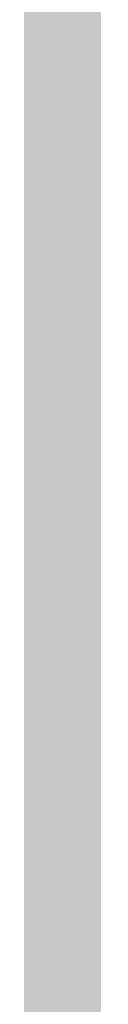
# Model space of a CAD drawing. Units: inches. Extents: x 2083 to 3317, y 1141 to 2115.
# Tile 228 of 256: x 3126.67 to 3126.939, y 1267.234 to 1271.372. Entities that reach past the tile are written whole.
import ezdxf

# ---------------------------------------------------------------- set-up
doc = ezdxf.new("R2010")
doc.units = ezdxf.units.IN
doc.layers.add('A-ANNO-DIMS', color=2, linetype='Continuous', lineweight=18)
doc.layers.add('A-WALL-PATT', color=251, linetype='Continuous', lineweight=13, true_color=0x636466)
doc.styles.get("Standard").update_dxf_attribs({"font": 'arial.ttf'})
doc.dimstyles.new('ISO-25', dxfattribs={"dimtxt": 12, "dimasz": 12, "dimexe": 1.25, "dimexo": 0.625, "dimtad": 1, "dimlunit": 3, "dimtxsty": 'Standard', "dimcen": 2.5, "dimadec": 0, "dimazin": 0, "dimtfac": 1, "dimtmove": 0, "dimatfit": 3, "dimfxl": 1, "dimarcsym": 0})

# ---------------------------------------------------------------- blocks, each defined once
blk = doc.blocks.new('*D26')
at = {"layer": 'A-ANNO-DIMS', "color": 0, "lineweight": -2, "transparency": 16777216}
for p, q in [((3088.9858, 1274.9151), (3088.9858, 1270.952)), ((3111.24, 1274.9151), (3111.24, 1270.952)), ((3076.9858, 1272.202), (2840.2624, 1272.202)), ((3111.24, 1272.202), (3088.9858, 1272.202)), ((3123.24, 1272.202), (3135.24, 1272.202))]:
    blk.add_line(p, q, dxfattribs=at)
at = {"layer": 'A-ANNO-DIMS', "color": 0, "transparency": 16777216}
for points in [[(3076.9858, 1274.202), (3076.9858, 1270.202), (3088.9858, 1272.202)], [(3123.24, 1274.202), (3123.24, 1270.202), (3111.24, 1272.202)]]:
    blk.add_solid(points, dxfattribs=at)
at = {"layer": 'Defpoints', "color": 0, "transparency": 16777216}
for p in [(3088.9858, 1275.5401), (3111.24, 1275.5401), (3088.9858, 1272.202)]:
    blk.add_point(p, dxfattribs=at)
at = {"layer": 'A-ANNO-DIMS', "color": 0, "transparency": 16777216, "insert": (2952.6241, 1279.0316), "char_height": 12, "attachment_point": 5}
blk.add_mtext('NIGHTSTAND 1\'-10 1/2" TYP.', dxfattribs=at)
blk = doc.blocks.new('*D27')
at = {"layer": 'A-ANNO-DIMS', "color": 0, "lineweight": -2, "transparency": 16777216}
for p, q in [((3114.5782, 1309.7943), (3114.5782, 1321.7943)), ((3111.865, 1297.7943), (3115.8282, 1297.7943)), ((3114.5782, 1297.7943), (3114.5782, 1275.5401)), ((3111.865, 1275.5401), (3115.8282, 1275.5401)), ((3114.5782, 1263.5401), (3114.5782, 1140.9886))]:
    blk.add_line(p, q, dxfattribs=at)
at = {"layer": 'A-ANNO-DIMS', "color": 0, "transparency": 16777216}
for points in [[(3112.5782, 1309.7943), (3116.5782, 1309.7943), (3114.5782, 1297.7943)], [(3112.5782, 1263.5401), (3116.5782, 1263.5401), (3114.5782, 1275.5401)]]:
    blk.add_solid(points, dxfattribs=at)
at = {"layer": 'Defpoints', "color": 0, "transparency": 16777216}
for p in [(3111.24, 1297.7943), (3111.24, 1275.5401), (3114.5782, 1275.5401)]:
    blk.add_point(p, dxfattribs=at)
at = {"layer": 'A-ANNO-DIMS', "color": 0, "transparency": 16777216, "insert": (3107.7485, 1196.2643), "char_height": 12, "attachment_point": 5, "rotation": 90}
blk.add_mtext('1\'-10 1/2" TYP.', dxfattribs=at)

msp = doc.modelspace()

# ---------------------------------------------------------------- hatches: boundary and pattern name
at = {"layer": 'A-WALL-PATT'}
h = msp.add_hatch(color=256, dxfattribs=at)
h.dxf.hatch_style = 1
h.paths.add_polyline_path([(3126.9598, 2020.7614), (2748.9598, 2020.7614), (2604.9598, 2020.7614), (2226.9598, 2020.7614), (2226.9598, 1702.7614), (2466.9598, 1702.7614), (2466.9598, 1582.7614), (2418.9598, 1582.7614), (2418.9598, 1477.7614), (2226.9598, 1477.7614), (2226.9598, 1263.2614), (2544.9598, 1263.2614), (2544.9598, 1411.7614), (2604.9598, 1411.7614), (2685.9598, 1411.7614), (2685.9598, 1420.7614), (2604.9598, 1420.7614), (2604.9598, 1573.7614), (2604.9598, 1702.7614), (2604.9598, 2011.7614), (2748.9598, 2011.7614), (2748.9598, 1702.7614), (2862.9598, 1702.7614), (2862.9598, 1621.7614), (2871.9598, 1621.7614), (2871.9598, 1702.7614), (2883.9598, 1702.7614), (2883.9598, 1706.9395, -0.026459), (2883.9598, 1711.7614), (2757.9598, 1711.7614), (2757.9598, 1807.7614), (2787.9598, 1807.7614), (2787.9598, 1812.2614), (2757.9598, 1812.2614), (2757.9598, 2011.7614), (2877.9598, 2011.7614), (2877.9598, 1812.2614), (2847.9598, 1812.2614), (2847.9598, 1807.7614), (2889.8357, 1807.7614), (2889.8357, 1812.2614), (2882.4598, 1812.2614), (2882.4598, 2011.7614), (3117.9598, 2011.7614), (3117.9598, 1812.2614), (2937.8357, 1812.2614), (2937.8357, 1807.7614), (2995.7098, 1807.7614), (2995.7098, 1796.1177), (3000.2098, 1796.1177), (3000.2098, 1807.7614), (3117.9598, 1807.7614), (3117.9598, 1711.7614), (3000.2098, 1711.7614), (3000.2098, 1760.1177), (2998.5727, 1760.1177, -0.020711), (2995.7098, 1760.1177), (2995.7098, 1711.7614), (2931.9598, 1711.7614), (2931.9598, 1702.7614), (3126.9598, 1702.7614)])
h.paths.add_polyline_path([(2471.4598, 2011.7614), (2471.4598, 1810.0114), (2462.7169, 1810.0114), (2462.7169, 1805.5114), (2505.9598, 1805.5114), (2505.9598, 1810.0114), (2475.9598, 1810.0114), (2475.9598, 2011.7614), (2595.9598, 2011.7614), (2595.9598, 1810.0114), (2565.9598, 1810.0114), (2565.9598, 1805.5114), (2595.9598, 1805.5114), (2595.9598, 1711.7614), (2235.9598, 1711.7614), (2235.9598, 1805.5114), (2353.7098, 1805.5114), (2353.7098, 1796.0542), (2358.2098, 1796.0542), (2358.2098, 1805.5114), (2414.7169, 1805.5114), (2414.7169, 1810.0114), (2235.9598, 1810.0114), (2235.9598, 2011.7614)], flags=16)
h.paths.add_polyline_path([(2270.2047, 1994.61), (2270.2047, 1970.61), (2246.2047, 1970.61), (2246.2047, 1994.61)], flags=0)
edge = h.paths.add_edge_path(flags=0)
edge.add_ellipse((2332.0274, 1899.7982), major_axis=(-3.043, 3.043), ratio=0.168252, start_angle=-161.3322, end_angle=-156.3071, ccw=False)
edge.add_ellipse((2333.082, 1898.7435), major_axis=(-1.0546, 1.0546), ratio=0.453532, start_angle=-123.371, end_angle=-94.1591)
edge = h.paths.add_edge_path(flags=0)
edge.add_ellipse((2332.0274, 1968.8763), major_axis=(3.043, 3.043), ratio=0.168252, start_angle=18.6678, end_angle=23.6929)
edge.add_spline(control_points=[(2332.9256, 1970.6911), (2332.2268, 1970.3361), (2330.8937, 1969.6589), (2328.4131, 1970.9321), (2327.2039, 1967.7487), (2324.7096, 1969.9556), (2322.5328, 1967.0124), (2320.0128, 1971.2958), (2317.6803, 1968.1578), (2316.0405, 1967.102), (2315.4269, 1966.8096)], knot_values=[0, 0, 0, 0, 2.267059, 4.324559, 6.685584, 8.878641, 11.121502, 14.300359, 17.755284, 19.732645, 19.732645, 19.732645, 19.732645], degree=3, periodic=0)
edge.add_ellipse((2332.0274, 1968.8763), major_axis=(3.043, 3.043), ratio=0.168252, start_angle=18.6678, end_angle=23.6929, ccw=False)
edge.add_ellipse((2333.082, 1969.9309), major_axis=(1.0546, 1.0546), ratio=0.453532, start_angle=56.629, end_angle=85.8409, ccw=False)
edge = h.paths.add_edge_path(flags=0)
edge.add_spline(control_points=[(2296.4283, 1967.9879), (2293.6278, 1965.3363), (2287.7036, 1959.7271), (2299.7439, 1949.9957), (2294.5326, 1935.6685), (2290.5732, 1920.6035), (2293.3941, 1909.9737), (2296.1854, 1904.9665)], knot_values=[0.099185, 0.099185, 0.099185, 0.099185, 0.345301, 0.619822, 0.982653, 1.386093, 1.810555, 1.810555, 1.810555, 1.810555], degree=3, periodic=0)
edge.add_spline(control_points=[(2296.1854, 1904.9665), (2297.3836, 1902.6193), (2298.001, 1901.9493), (2298.553, 1901.4682)], knot_values=[0.006246, 0.006246, 0.006246, 0.006246, 0.055476, 0.055476, 0.055476, 0.055476], degree=3, periodic=0)
edge.add_spline(control_points=[(2298.553, 1901.4682), (2297.2586, 1900.9232), (2295.2253, 1900.2321), (2293.0602, 1900.6142), (2292.1014, 1900.7884), (2292.0896, 1900.7906)], knot_values=[0.312835, 0.312835, 0.312835, 0.312835, 0.40178, 0.474987, 0.475903, 0.475903, 0.475903, 0.475903], degree=3, periodic=0)
edge.add_arc((2292.7936, 1904.6641), 3.937, 215.4209, 259.6982, ccw=False)
edge.add_spline(control_points=[(2289.5853, 1902.3823), (2289.4767, 1902.5351), (2289.3685, 1902.688), (2289.2609, 1902.8412)], knot_values=[0.102872, 0.102872, 0.102872, 0.102872, 0.116896, 0.116896, 0.116896, 0.116896], degree=3, periodic=0)
edge.add_spline(control_points=[(2289.2609, 1902.8412), (2288.6866, 1902.5502), (2287.64, 1902.0199), (2285.8813, 1901.874), (2283.853, 1901.5044), (2281.72, 1899.7105), (2278.467, 1899.4929), (2276.1571, 1901.8832), (2272.259, 1899.8041), (2267.7776, 1901.8432), (2262.2439, 1900.184), (2257.4149, 1901.7821), (2254.3184, 1900.7261), (2253.1783, 1900.3373)], knot_values=[0, 0, 0, 0, 1.907977, 3.477176, 5.261074, 7.972851, 11.680248, 13.717921, 16.939592, 22.789562, 27.502503, 33.595215, 37.145618, 37.145618, 37.145618, 37.145618], degree=3, periodic=0)
edge.add_line((2253.1783, 1900.3373), (2250.2442, 1902.8412))
edge.add_line((2250.2442, 1902.8412), (2250.2442, 1965.8333))
edge.add_line((2250.2442, 1965.8333), (2253.1783, 1968.3371))
edge.add_spline(control_points=[(2253.1783, 1968.3371), (2254.3184, 1967.9483), (2257.4149, 1966.8924), (2262.2439, 1968.4904), (2267.7776, 1966.8313), (2271.5267, 1968.5372), (2273.8759, 1967.8283), (2274.2067, 1967.7276)], knot_values=[0, 0, 0, 0, 0.09018, 0.244935, 0.364644, 0.513233, 0.537855, 0.537855, 0.537855, 0.537855], degree=3, periodic=0)
edge.add_arc((2274.3529, 1963.7933), 3.937, 72.0511, 92.1279, ccw=False)
edge.add_arc((2281.2969, 1985.23), 18.5963, 252.05113, 288.56572)
edge.add_arc((2292.3167, 1956.0289), 12.6461, 71.02679, 113.77822, ccw=False)
edge = h.paths.add_edge_path(flags=0)
edge.add_spline(control_points=[(2274.8994, 1951.8562), (2275.0662, 1951.6166), (2275.2327, 1951.3766), (2275.398, 1951.1359)], knot_values=[1.409916, 1.409916, 1.409916, 1.409916, 1.43159, 1.43159, 1.43159, 1.43159], degree=3, periodic=0)
edge.add_spline(control_points=[(2275.398, 1951.1359), (2275.7921, 1950.5619), (2276.1792, 1949.9838), (2276.5455, 1949.3971)], knot_values=[1.358238, 1.358238, 1.358238, 1.358238, 1.409916, 1.409916, 1.409916, 1.409916], degree=3, periodic=0)
edge.add_line((2276.5455, 1949.3971), (2277.4373, 1947.8622))
edge.add_spline(control_points=[(2277.4373, 1947.8622), (2276.3038, 1945.6731), (2274.6397, 1942.4269), (2274.6316, 1938.0939), (2272.7991, 1930.8515), (2274.3564, 1943.897), (2275.9477, 1947.9234), (2276.5455, 1949.3971)], knot_values=[0.005632, 0.005632, 0.005632, 0.005632, 0.186014, 0.266002, 0.357087, 0.59639, 0.739732, 0.739732, 0.739732, 0.739732], degree=3, periodic=0)
edge.add_spline(control_points=[(2276.5455, 1949.3971), (2276.1792, 1949.9838), (2275.7921, 1950.5619), (2275.398, 1951.1359)], knot_values=[1.358238, 1.358238, 1.358238, 1.358238, 1.409916, 1.409916, 1.409916, 1.409916], degree=3, periodic=0)
edge.add_spline(control_points=[(2275.398, 1951.1359), (2274.9425, 1950.0805), (2274.2078, 1948.0253), (2273.9346, 1944.8515), (2272.4685, 1937.6275), (2273.4662, 1945.6965), (2274.7006, 1951.0595), (2274.8994, 1951.8562)], knot_values=[0.104364, 0.104364, 0.104364, 0.104364, 0.189636, 0.269624, 0.36071, 0.600013, 0.644622, 0.644622, 0.644622, 0.644622], degree=3, periodic=0)
h.paths.add_polyline_path([(2269.1675, 1963.1276, -0.357527), (2268.1706, 1960.9764, -0.092561), (2268.1706, 1939.4363, -0.357527), (2269.1675, 1937.2851, -0.357527), (2267.0163, 1938.282, -0.164785), (2254.6856, 1938.282, -0.357527), (2252.5344, 1937.2851, -0.357527), (2253.5313, 1939.4363, -0.092561), (2253.5313, 1960.9764, -0.357527), (2252.5344, 1963.1276, -0.357527), (2254.6856, 1962.1307, -0.164785), (2267.0163, 1962.1307, -0.357527)], flags=0)
h.paths.add_polyline_path([(2248.8741, 1967.8018), (2248.8741, 1957.0277), (2249.4578, 1957.0277), (2249.4578, 1911.6468), (2248.8741, 1911.6468), (2248.8741, 1900.8727), (2246.5119, 1900.8727, 0.197327), (2244.1497, 1902.4569), (2244.1497, 1966.2176, 0.197327), (2246.5119, 1967.8018)], flags=0)
h.paths.add_polyline_path([(2269.1675, 1931.3893, -0.357527), (2268.1706, 1929.2381, -0.092561), (2268.1706, 1907.6981, -0.357527), (2269.1675, 1905.5469, -0.357527), (2267.0163, 1906.5438, -0.164785), (2254.6856, 1906.5438, -0.357527), (2252.5344, 1905.5469, -0.357527), (2253.5313, 1907.6981, -0.092561), (2253.5313, 1929.2381, -0.357527), (2252.5344, 1931.3893, -0.357527), (2254.6856, 1930.3925, -0.164785), (2267.0163, 1930.3925, -0.357527)], flags=0)
edge = h.paths.add_edge_path(flags=0)
edge.add_spline(control_points=[(2276.1969, 1906.7237), (2276.1681, 1909.0289), (2276.114, 1913.3719), (2270.5984, 1924.925), (2273.9052, 1919.0128), (2275.9217, 1916.2621), (2275.4746, 1912.4021), (2277.2579, 1910.3806), (2276.696, 1908.225), (2276.6462, 1906.813), (2276.6178, 1906.0084)], knot_values=[0, 0, 0, 0, 8.61026, 16.221274, 18.843057, 23.804898, 27.440828, 29.356102, 31.203478, 33.650687, 33.650687, 33.650687, 33.650687], degree=3, periodic=0)
edge.add_spline(control_points=[(2276.6178, 1906.0084), (2276.6233, 1905.6241), (2276.4977, 1904.6287), (2275.4418, 1903.8547), (2274.9373, 1903.0804), (2274.8591, 1902.8412)], knot_values=[0.156488, 0.156488, 0.156488, 0.156488, 0.184398, 0.231376, 0.250598, 0.250598, 0.250598, 0.250598], degree=3, periodic=0)
edge.add_line((2274.8591, 1902.8412), (2276.506, 1902.8412))
edge.add_spline(control_points=[(2276.506, 1902.8412), (2276.7883, 1903.0849), (2277.6651, 1904.1252), (2278.2495, 1904.3407), (2277.6539, 1908.5274), (2278.1557, 1906.2278), (2278.1005, 1905.2859), (2278.8467, 1904.069), (2277.8568, 1903.4149), (2277.8742, 1902.991), (2277.9036, 1902.8412)], knot_values=[0.059574, 0.059574, 0.059574, 0.059574, 0.080753, 0.103741, 0.16972, 0.176036, 0.207137, 0.240474, 0.262341, 0.27366, 0.27366, 0.27366, 0.27366], degree=3, periodic=0)
edge.add_line((2277.9036, 1902.8412), (2280.0298, 1902.8412))
edge.add_spline(control_points=[(2280.0298, 1902.8412), (2279.8882, 1903.0884), (2279.4993, 1903.9816), (2280.1523, 1905.9393), (2278.1036, 1909.6578), (2279.7624, 1907.1853), (2280.3279, 1904.8749), (2280.4851, 1903.4896), (2281.4633, 1903.2494), (2281.7583, 1902.9365), (2281.834, 1902.8412)], knot_values=[0.013856, 0.013856, 0.013856, 0.013856, 0.034874, 0.088867, 0.107879, 0.126738, 0.158714, 0.193757, 0.217487, 0.226722, 0.226722, 0.226722, 0.226722], degree=3, periodic=0)
edge.add_spline(control_points=[(2281.834, 1902.8412), (2281.7875, 1902.8267), (2281.647, 1902.783), (2281.3955, 1902.8595), (2281.0881, 1902.9852), (2280.7207, 1903.0609), (2280.3335, 1903.0257), (2280.1248, 1902.8989), (2280.0298, 1902.8412)], knot_values=[0, 0, 0, 0, 0.14413, 0.435517, 0.749276, 1.153046, 1.548371, 1.878348, 1.878348, 1.878348, 1.878348], degree=3, periodic=0)
edge.add_line((2280.0298, 1902.8412), (2277.9036, 1902.8412))
edge.add_spline(control_points=[(2277.9036, 1902.8412), (2277.8929, 1902.7959), (2277.8654, 1902.6796), (2277.6075, 1902.6875), (2277.2741, 1902.8007), (2276.8379, 1902.6198), (2276.5838, 1902.7893), (2276.506, 1902.8412)], knot_values=[0, 0, 0, 0, 0.127189, 0.326199, 0.628009, 1.24357, 1.515331, 1.515331, 1.515331, 1.515331], degree=3, periodic=0)
edge.add_line((2276.506, 1902.8412), (2274.8591, 1902.8412))
edge.add_spline(control_points=[(2274.8591, 1902.8412), (2274.8144, 1902.8986), (2274.7251, 1903.0134), (2274.4935, 1903.119), (2274.2443, 1902.9605), (2273.9371, 1903.1849), (2273.614, 1902.9831), (2273.4083, 1902.883), (2273.3223, 1902.8412)], knot_values=[0, 0, 0, 0, 0.21843, 0.436957, 0.687977, 0.990379, 1.398396, 1.69185, 1.69185, 1.69185, 1.69185], degree=3, periodic=0)
edge.add_spline(control_points=[(2273.3223, 1902.8412), (2273.6167, 1903.4457), (2274.274, 1904.5383), (2276.0272, 1904.5737), (2276.207, 1906.5836), (2276.1969, 1906.7237)], knot_values=[0.012227, 0.012227, 0.012227, 0.012227, 0.059472, 0.106218, 0.134458, 0.134458, 0.134458, 0.134458], degree=3, periodic=0)
h.paths.add_polyline_path([(2270.7761, 1897.7898), (2270.7761, 1873.7898), (2246.7761, 1873.7898), (2246.7761, 1897.7898)], flags=0)
h.paths.add_polyline_path([(2353.7098, 1760.0051), (2353.7098, 1760.0542), (2358.2098, 1760.0542, -0.033729)], flags=0)
h.paths.add_polyline_path([(2321.8191, 1737.5292), (2341.9953, 1737.5292, -0.414214), (2343.2033, 1736.3212), (2343.2033, 1721.0206, -0.414214), (2341.9953, 1719.8127), (2321.8191, 1719.8127, -0.414214), (2320.6112, 1721.0206), (2320.6112, 1736.3212, -0.414214)], flags=0)
h.paths.add_polyline_path([(2324.235, 1736.3212), (2339.5794, 1736.3212, -0.414214), (2341.9953, 1733.9053), (2341.9953, 1725.4497, -0.414214), (2339.5794, 1723.0338), (2333.6806, 1723.0338), (2333.8453, 1722.0455, -0.870646), (2335.4254, 1721.8259, -0.767327), (2333.9227, 1721.4232), (2331.291, 1721.4232, -0.767327), (2329.7883, 1721.8259, -0.870646), (2331.3684, 1722.0455), (2331.5331, 1723.0338), (2324.235, 1723.0338, -0.414214), (2321.8191, 1725.4497), (2321.8191, 1733.9053, -0.414214)], flags=0)
h.paths.add_polyline_path([(2570.4838, 1928.6154), (2589.6838, 1928.6154), (2590.1688, 1928.6154), (2590.1688, 1904.9934), (2570.4838, 1904.9934)], flags=0)
h.paths.add_polyline_path([(2574.4473, 1927.2638, -1), (2572.8288, 1927.2638, -1)], flags=0)
h.paths.add_polyline_path([(2573.0899, 1926.9409), (2573.925, 1927.776), (2574.1477, 1927.5533), (2573.3126, 1926.7182)], flags=0)
h.paths.add_polyline_path([(2578.7791, 1919.7296, -1), (2571.5917, 1919.7296, -1)], flags=0)
h.paths.add_polyline_path([(2578.3854, 1919.7296, -1), (2571.9854, 1919.7296, -1)], flags=0)
h.paths.add_polyline_path([(2331.5958, 1729.4762, -1), (2333.618, 1729.4762, -1)], flags=0)
h.paths.add_polyline_path([(2578.0342, 1927.2638, -1), (2576.4157, 1927.2638, -1)], flags=0)
h.paths.add_polyline_path([(2576.6889, 1927.5311), (2576.9116, 1927.7538), (2577.7467, 1926.9186), (2577.524, 1926.6959)], flags=0)
h.paths.add_polyline_path([(2578.1391, 1909.8595, -1), (2572.2317, 1909.8595, -1)], flags=0)
h.paths.add_polyline_path([(2577.7454, 1909.8595, -1), (2572.6254, 1909.8595, -1)], flags=0)
h.paths.add_polyline_path([(2583.7977, 1927.2638, -1), (2582.1792, 1927.2638, -1)], flags=0)
h.paths.add_polyline_path([(2582.7186, 1927.7538), (2583.5538, 1926.9186), (2583.3311, 1926.6959), (2582.4959, 1927.5311)], flags=0)
h.paths.add_polyline_path([(2582.4959, 1927.5311), (2582.7186, 1927.7538), (2583.5538, 1926.9186), (2583.3311, 1926.6959)], flags=0)
h.paths.add_polyline_path([(2587.7391, 1920.5296, -1), (2581.8317, 1920.5296, -1)], flags=0)
h.paths.add_polyline_path([(2587.3454, 1920.5296, -1), (2582.2254, 1920.5296, -1)], flags=0)
h.paths.add_polyline_path([(2587.3846, 1927.2638, -1), (2585.7661, 1927.2638, -1)], flags=0)
h.paths.add_polyline_path([(2586.082, 1926.9802), (2586.9172, 1927.8154), (2587.1399, 1927.5927), (2586.3047, 1926.7575)], flags=0)
h.paths.add_polyline_path([(2588.3791, 1910.6595, -1), (2581.1917, 1910.6595, -1)], flags=0)
h.paths.add_polyline_path([(2587.9854, 1910.6595, -1), (2581.5854, 1910.6595, -1)], flags=0)
h.paths.add_polyline_path([(2417.1677, 1729.4779), (2437.3439, 1729.4779, -0.414214), (2438.5519, 1728.2699), (2438.5519, 1712.9693, -0.414214), (2437.3439, 1711.7614), (2417.1677, 1711.7614, -0.414214), (2415.9598, 1712.9693), (2415.9598, 1728.2699, -0.414214)], flags=0)
h.paths.add_polyline_path([(2419.5836, 1728.2699), (2434.928, 1728.2699, -0.414214), (2437.3439, 1725.8541), (2437.3439, 1717.3984, -0.414214), (2434.928, 1714.9825), (2429.0292, 1714.9825), (2429.1939, 1713.9942, -0.870646), (2430.774, 1713.7746, -0.767327), (2429.2713, 1713.372), (2426.6396, 1713.372, -0.767327), (2425.1369, 1713.7746, -0.870646), (2426.717, 1713.9942), (2426.8817, 1714.9825), (2419.5836, 1714.9825, -0.414214), (2417.1677, 1717.3984), (2417.1677, 1725.8541, -0.414214)], flags=0)
h.paths.add_polyline_path([(2419.5836, 1728.2699), (2434.928, 1728.2699, -0.414214), (2437.3439, 1725.8541), (2437.3439, 1717.3984, -0.414214), (2434.928, 1714.9825), (2429.0292, 1714.9825), (2428.3581, 1719.009), (2427.5528, 1719.009), (2426.8817, 1714.9825), (2419.5836, 1714.9825, -0.414214), (2417.1677, 1717.3984), (2417.1677, 1725.8541, -0.414214)], flags=0)
h.paths.add_polyline_path([(2426.9444, 1721.4249, -1), (2428.9666, 1721.4249, -1)], flags=0)
h.paths.add_polyline_path([(2475.9598, 1702.7614), (2595.9598, 1702.7614), (2595.9598, 1582.7614), (2475.9598, 1582.7614)], flags=16)
h.paths.add_polyline_path([(2427.9598, 1573.7614), (2595.9598, 1573.7614), (2595.9598, 1468.7614), (2595.9598, 1420.7614), (2384.4598, 1420.7614), (2384.4598, 1468.7614), (2427.9598, 1468.7614)], flags=16)
h.paths.add_polyline_path([(2379.9598, 1468.7614), (2379.9598, 1420.7614), (2235.9598, 1420.7614), (2235.9598, 1468.7614)], flags=16)
h.paths.add_polyline_path([(2317.816, 1466.6958), (2337.9922, 1466.6958, -0.414214), (2339.2002, 1465.4878), (2339.2002, 1450.1872, -0.414214), (2337.9922, 1448.9792), (2317.816, 1448.9792, -0.414214), (2316.6081, 1450.1872), (2316.6081, 1465.4878, -0.414214)], flags=0)
h.paths.add_polyline_path([(2320.2319, 1465.4878), (2335.5763, 1465.4878, -0.414214), (2337.9922, 1463.0719), (2337.9922, 1454.6163, -0.414214), (2335.5763, 1452.2004), (2329.6775, 1452.2004), (2329.8422, 1451.212, -0.870646), (2331.4223, 1450.9925, -0.767327), (2329.9196, 1450.5898), (2327.2879, 1450.5898, -0.767327), (2325.7852, 1450.9925, -0.870646), (2327.3653, 1451.212), (2327.53, 1452.2004), (2320.2319, 1452.2004, -0.414214), (2317.816, 1454.6163), (2317.816, 1463.0719, -0.414214)], flags=0)
h.paths.add_polyline_path([(2320.2319, 1465.4878), (2335.5763, 1465.4878, -0.414214), (2337.9922, 1463.0719), (2337.9922, 1454.6163, -0.414214), (2335.5763, 1452.2004), (2329.6775, 1452.2004), (2329.0064, 1456.2269), (2328.2011, 1456.2269), (2327.53, 1452.2004), (2320.2319, 1452.2004, -0.414214), (2317.816, 1454.6163), (2317.816, 1463.0719, -0.414214)], flags=0)
h.paths.add_polyline_path([(2327.5926, 1458.6428, -1), (2329.6148, 1458.6428, -1)], flags=0)
h.paths.add_polyline_path([(2244.4117, 1433.3405), (2241.9209, 1433.3405, -0.414214), (2240.0179, 1435.2435), (2240.0179, 1440.9528, -0.414211), (2241.9209, 1442.8559), (2244.4117, 1442.8559, -1.976472)], flags=0)
h.paths.add_polyline_path([(2245.3569, 1434.3975, -0.414214), (2245.3569, 1441.7988, -2.144098)], flags=0)
h.paths.add_polyline_path([(2535.9598, 1416.2614), (2535.9598, 1272.2614), (2235.9598, 1272.2614), (2235.9598, 1416.2614)], flags=16)
h.paths.add_polyline_path([(2260.1196, 1384.2928), (2260.1196, 1362.0386), (2237.8654, 1362.0386), (2237.8654, 1384.2928)], flags=0)
edge = h.paths.add_edge_path(flags=0)
edge.add_line((2318.2518, 1362.0933), (2318.1458, 1362.001))
edge.add_ellipse((2317.4451, 1360.431), major_axis=(2.8216, 2.8216), ratio=0.168252, start_angle=18.6678, end_angle=20.9481, ccw=False)
edge.add_ellipse((2318.423, 1361.409), major_axis=(0.9779, 0.9779), ratio=0.453532, start_angle=56.629, end_angle=70.2262, ccw=False)
edge = h.paths.add_edge_path(flags=0)
edge.add_line((2319.1074, 1295.5711), (2319.015, 1295.6771))
edge.add_ellipse((2317.4451, 1296.3778), major_axis=(-2.8216, 2.8216), ratio=0.168252, start_angle=-161.3322, end_angle=-159.0519, ccw=False)
edge.add_ellipse((2318.423, 1295.3999), major_axis=(-0.9779, 0.9779), ratio=0.453532, start_angle=-123.371, end_angle=-109.7738)
edge = h.paths.add_edge_path(flags=0)
edge.add_spline(control_points=[(2284.2103, 1301.1702), (2284.5807, 1300.4447), (2284.8912, 1299.892), (2285.1596, 1299.461)], knot_values=[0.039066, 0.039066, 0.039066, 0.039066, 0.055476, 0.055476, 0.055476, 0.055476], degree=3, periodic=0)
edge.add_line((2285.1596, 1299.461), (2284.2103, 1301.1702))
edge = h.paths.add_edge_path(flags=0)
edge.add_line((2280.4125, 1297.298), (2283.37, 1297.0361))
edge.add_line((2283.37, 1297.0361), (2286.4057, 1297.9263))
edge.add_spline(control_points=[(2286.4057, 1297.9263), (2285.3055, 1297.4631), (2284.3448, 1297.1292), (2283.37, 1297.0361)], knot_values=[0.394369, 0.394369, 0.394369, 0.394369, 0.475903, 0.475903, 0.475903, 0.475903], degree=3, periodic=0)
edge.add_spline(control_points=[(2283.37, 1297.0361), (2283.2814, 1297.0277), (2282.3163, 1296.9573), (2281.3125, 1297.1345), (2280.4234, 1297.296), (2280.4125, 1297.298)], knot_values=[0.312835, 0.312835, 0.312835, 0.312835, 0.320246, 0.393453, 0.394369, 0.394369, 0.394369, 0.394369], degree=3, periodic=0)
edge = h.paths.add_edge_path(flags=0)
edge.add_line((2284.4356, 1359.6073), (2280.4463, 1355.328))
edge.add_line((2280.4463, 1355.328), (2279.58, 1351.0178))
edge.add_line((2279.58, 1351.0178), (2282.413, 1346.5804))
edge.add_spline(control_points=[(2282.413, 1346.5804), (2283.1533, 1345.5892), (2284.2529, 1344.0289), (2284.801, 1342.3872), (2284.9352, 1341.8055)], knot_values=[1.240098, 1.240098, 1.240098, 1.240098, 1.332892, 1.382712, 1.382712, 1.382712, 1.382712], degree=3, periodic=0)
edge.add_spline(control_points=[(2284.9352, 1341.8055), (2285.3191, 1340.1406), (2285.233, 1338.4092), (2284.9099, 1336.6541)], knot_values=[1.097484, 1.097484, 1.097484, 1.097484, 1.240098, 1.240098, 1.240098, 1.240098], degree=3, periodic=0)
edge.add_spline(control_points=[(2284.9099, 1336.6541), (2284.5868, 1334.899), (2284.0267, 1333.1203), (2283.4626, 1331.3606)], knot_values=[0.95487, 0.95487, 0.95487, 0.95487, 1.097484, 1.097484, 1.097484, 1.097484], degree=3, periodic=0)
edge.add_line((2283.4626, 1331.3606), (2281.8904, 1326.1534))
edge.add_line((2281.8904, 1326.1534), (2280.7563, 1321.0561))
edge.add_line((2280.7563, 1321.0561), (2280.2992, 1316.002))
edge.add_line((2280.2992, 1316.002), (2280.7159, 1310.9501))
edge.add_line((2280.7159, 1310.9501), (2282.0281, 1305.9721))
edge.add_line((2282.0281, 1305.9721), (2284.2103, 1301.1702))
edge.add_spline(control_points=[(2284.2103, 1301.1702), (2283.3407, 1302.7302), (2282.6119, 1304.3365), (2282.0281, 1305.9721)], knot_values=[0.099185, 0.099185, 0.099185, 0.099185, 0.241799, 0.241799, 0.241799, 0.241799], degree=3, periodic=0)
edge.add_spline(control_points=[(2282.0281, 1305.9721), (2281.4443, 1307.6078), (2281.0055, 1309.2728), (2280.7159, 1310.9501)], knot_values=[0.241799, 0.241799, 0.241799, 0.241799, 0.384413, 0.384413, 0.384413, 0.384413], degree=3, periodic=0)
edge.add_spline(control_points=[(2280.7159, 1310.9501), (2280.4332, 1312.5876), (2280.2894, 1314.277), (2280.2989, 1315.962), (2280.2992, 1316.002)], knot_values=[0.384413, 0.384413, 0.384413, 0.384413, 0.523647, 0.527028, 0.527028, 0.527028, 0.527028], degree=3, periodic=0)
edge.add_spline(control_points=[(2280.2992, 1316.002), (2280.3123, 1317.687), (2280.4779, 1319.3679), (2280.7563, 1321.0561)], knot_values=[0.527028, 0.527028, 0.527028, 0.527028, 0.669642, 0.669642, 0.669642, 0.669642], degree=3, periodic=0)
edge.add_spline(control_points=[(2280.7563, 1321.0561), (2281.0346, 1322.7443), (2281.4259, 1324.4396), (2281.8904, 1326.1534)], knot_values=[0.669642, 0.669642, 0.669642, 0.669642, 0.812256, 0.812256, 0.812256, 0.812256], degree=3, periodic=0)
edge.add_spline(control_points=[(2281.8904, 1326.1534), (2282.2644, 1327.5333), (2282.7879, 1329.2618), (2283.3528, 1331.0178), (2283.4626, 1331.3606)], knot_values=[0.812256, 0.812256, 0.812256, 0.812256, 0.927087, 0.95487, 0.95487, 0.95487, 0.95487], degree=3, periodic=0)
edge.add_line((2283.4626, 1331.3606), (2284.9099, 1336.6541))
edge.add_line((2284.9099, 1336.6541), (2284.9352, 1341.8055))
edge.add_line((2284.9352, 1341.8055), (2282.413, 1346.5804))
edge.add_spline(control_points=[(2282.413, 1346.5804), (2281.2751, 1348.1038), (2280.0784, 1349.5703), (2279.58, 1351.0178)], knot_values=[1.382712, 1.382712, 1.382712, 1.382712, 1.525326, 1.525326, 1.525326, 1.525326], degree=3, periodic=0)
edge.add_spline(control_points=[(2279.58, 1351.0178), (2279.4433, 1351.4147), (2279.1363, 1352.8569), (2279.7352, 1354.2904), (2280.4463, 1355.328)], knot_values=[1.525326, 1.525326, 1.525326, 1.525326, 1.564439, 1.667941, 1.667941, 1.667941, 1.667941], degree=3, periodic=0)
edge.add_spline(control_points=[(2280.4463, 1355.328), (2281.4261, 1356.7578), (2282.9308, 1358.1826), (2284.4356, 1359.6073)], knot_values=[1.667941, 1.667941, 1.667941, 1.667941, 1.810555, 1.810555, 1.810555, 1.810555], degree=3, periodic=0)
edge.add_arc((2280.6231, 1348.5182), 11.7262, 71.02679, 113.77822)
edge.add_arc((2270.4049, 1375.5952), 17.2436, 252.05113, 288.56572, ccw=False)
edge.add_arc((2263.966, 1355.7178), 3.6506, 72.0511, 92.1279)
edge.add_arc((2263.966, 1355.7178), 3.6506, 92.1279, 177.9851)
edge.add_spline(control_points=[(2260.3176, 1355.8462), (2260.2604, 1354.2207), (2260.5513, 1350.1865), (2262.9993, 1346.7663), (2264.4727, 1344.649)], knot_values=[1.43159, 1.43159, 1.43159, 1.43159, 1.564144, 1.770695, 1.770695, 1.770695, 1.770695], degree=3, periodic=0)
edge.add_line((2264.4727, 1344.649), (2264.9356, 1343.9825))
edge.add_spline(control_points=[(2263.801, 1340.2481), (2263.8432, 1340.5141), (2264.0672, 1341.7565), (2264.5127, 1343.0025), (2264.935, 1343.9811)], knot_values=[0.53657, 0.53657, 0.53657, 0.53657, 0.559349, 0.644622, 0.644622, 0.644622, 0.644622], degree=3, periodic=0)
edge.add_spline(control_points=[(2264.935, 1343.9811), (2265.1178, 1343.715), (2265.2989, 1343.4479), (2265.4768, 1343.1794)], knot_values=[1.384077, 1.384077, 1.384077, 1.384077, 1.409916, 1.409916, 1.409916, 1.409916], degree=3, periodic=0)
edge.add_spline(control_points=[(2265.4768, 1343.1794), (2265.6546, 1342.9108), (2265.8293, 1342.6408), (2265.9991, 1342.3688)], knot_values=[1.358238, 1.358238, 1.358238, 1.358238, 1.384077, 1.384077, 1.384077, 1.384077], degree=3, periodic=0)
edge.add_line((2265.9991, 1342.3688), (2266.826, 1340.9455))
edge.add_spline(control_points=[(2266.826, 1340.9455), (2268.8944, 1337.0897), (2271.3982, 1325.843), (2270.5162, 1310.5686), (2275.9194, 1301.8606), (2277.7895, 1299.1994)], knot_values=[0.116896, 0.116896, 0.116896, 0.116896, 0.472987, 1.050969, 1.313793, 1.313793, 1.313793, 1.313793], degree=3, periodic=0)
edge.add_spline(control_points=[(2277.7895, 1299.1994), (2277.8394, 1299.1285), (2277.8894, 1299.0575), (2277.9396, 1298.9866)], knot_values=[0.109884, 0.109884, 0.109884, 0.109884, 0.116896, 0.116896, 0.116896, 0.116896], degree=3, periodic=0)
edge.add_line((2277.9396, 1298.9866), (2277.7888, 1299.1991))
edge.add_spline(control_points=[(2277.7888, 1299.1991), (2277.2566, 1298.9294), (2276.2864, 1298.4379), (2275.0394, 1298.3344), (2274.3833, 1298.2389), (2274.2153, 1298.2093)], knot_values=[33.12187, 33.12187, 33.12187, 33.12187, 35.029056, 36.598255, 37.144827, 37.144827, 37.144827, 37.144827], degree=3, periodic=0)
edge.add_line((2274.2153, 1298.2093), (2273.0731, 1297.893))
edge.add_spline(control_points=[(2273.0731, 1297.893), (2272.3229, 1297.5798), (2271.0392, 1296.5105), (2269.2484, 1296.2261), (2268.4231, 1296.3747)], knot_values=[26.532584, 26.532584, 26.532584, 26.532584, 29.198919, 31.839101, 31.839101, 31.839101, 31.839101], degree=3, periodic=0)
edge.add_line((2268.4231, 1296.3747), (2263.8785, 1297.4575))
edge.add_spline(control_points=[(2263.8785, 1297.4575), (2263.5561, 1297.3594), (2261.8603, 1296.8387), (2260.2388, 1297.2824), (2258.9335, 1297.5165)], knot_values=[15.919551, 15.919551, 15.919551, 15.919551, 16.939592, 21.226067, 21.226067, 21.226067, 21.226067], degree=3, periodic=0)
edge.add_line((2258.9335, 1297.5165), (2254.0552, 1297.329))
edge.add_spline(control_points=[(2254.0552, 1297.329), (2253.7555, 1297.2958), (2252.1137, 1297.1652), (2250.4619, 1297.5442), (2249.1297, 1297.6679)], knot_values=[5.306517, 5.306517, 5.306517, 5.306517, 6.276435, 10.613034, 10.613034, 10.613034, 10.613034], degree=3, periodic=0)
edge.add_line((2249.1297, 1297.6679), (2244.3316, 1296.8778))
edge.add_line((2244.3316, 1296.8778), (2241.611, 1299.1994))
edge.add_line((2241.611, 1299.1994), (2241.611, 1357.6094))
edge.add_line((2241.611, 1357.6094), (2244.3316, 1359.9311))
edge.add_line((2244.3316, 1359.9311), (2252.7288, 1359.5427))
edge.add_spline(control_points=[(2252.7288, 1359.5427), (2252.8709, 1359.5464), (2253.3057, 1359.5482), (2253.7398, 1359.5143), (2254.0317, 1359.4824)], knot_values=[0.233291, 0.233291, 0.233291, 0.233291, 0.244935, 0.268927, 0.268927, 0.268927, 0.268927], degree=3, periodic=0)
edge.add_line((2254.0317, 1359.4824), (2259.5872, 1359.4164))
edge.add_spline(control_points=[(2259.5872, 1359.4164), (2260.6771, 1359.6285), (2262.0732, 1359.897), (2263.5237, 1359.4593), (2263.8304, 1359.366)], knot_values=[0.422516, 0.422516, 0.422516, 0.422516, 0.513233, 0.537855, 0.537855, 0.537855, 0.537855], degree=3, periodic=0)
edge.add_arc((2263.966, 1355.7178), 3.6506, 72.0511, 92.1279, ccw=False)
edge.add_arc((2270.4049, 1375.5952), 17.2436, 252.05113, 288.56572)
edge.add_arc((2280.6231, 1348.5182), 11.7262, 71.02679, 113.77822, ccw=False)
h.paths.add_polyline_path([(2240.3405, 1359.4347), (2240.3405, 1349.4444), (2240.8818, 1349.4444), (2240.8818, 1307.3645), (2240.3405, 1307.3645), (2240.3405, 1297.3741), (2238.1502, 1297.3741, 0.197327), (2235.9598, 1298.8431), (2235.9598, 1357.9657, 0.197327), (2238.1502, 1359.4347)], flags=0)
h.paths.add_polyline_path([(2259.1578, 1355.1005, -0.357527), (2258.2334, 1353.1058, -0.092561), (2258.2334, 1333.1326, -0.357527), (2259.1578, 1331.1379, -0.357527), (2257.1631, 1332.0622, -0.164785), (2245.7293, 1332.0622, -0.357527), (2243.7346, 1331.1379, -0.357527), (2244.6589, 1333.1326, -0.092561), (2244.6589, 1353.1058, -0.357527), (2243.7346, 1355.1005, -0.357527), (2245.7293, 1354.1761, -0.164785), (2257.1631, 1354.1761, -0.357527)], flags=0)
edge = h.paths.add_edge_path(flags=0)
edge.add_line((2265.9991, 1342.3688), (2266.826, 1340.9455))
edge.add_line((2266.826, 1340.9455), (2265.3076, 1337.8141))
edge.add_line((2265.3076, 1337.8141), (2264.3582, 1334.6529))
edge.add_line((2264.3582, 1334.6529), (2264.262, 1333.7997))
edge.add_spline(control_points=[(2264.262, 1333.7997), (2264.2084, 1333.1871), (2264.1621, 1332.3655), (2264.0071, 1331.4139), (2263.969, 1331.2018)], knot_values=[0.464444, 0.464444, 0.464444, 0.464444, 0.516691, 0.531608, 0.531608, 0.531608, 0.531608], degree=3, periodic=0)
edge.add_spline(control_points=[(2263.969, 1331.2018), (2263.7745, 1330.1189), (2263.4244, 1328.7908), (2263.2574, 1328.5307), (2263.234, 1328.5146)], knot_values=[0.372682, 0.372682, 0.372682, 0.372682, 0.44885, 0.464444, 0.464444, 0.464444, 0.464444], degree=3, periodic=0)
edge.add_spline(control_points=[(2263.234, 1328.5146), (2263.0964, 1328.4202), (2263.1312, 1329.3015), (2263.275, 1330.6157)], knot_values=[0.280919, 0.280919, 0.280919, 0.280919, 0.372682, 0.372682, 0.372682, 0.372682], degree=3, periodic=0)
edge.add_spline(control_points=[(2263.275, 1330.6157), (2263.4187, 1331.93), (2263.6715, 1333.6773), (2263.9699, 1335.315)], knot_values=[0.189157, 0.189157, 0.189157, 0.189157, 0.280919, 0.280919, 0.280919, 0.280919], degree=3, periodic=0)
edge.add_spline(control_points=[(2263.9699, 1335.315), (2264.1005, 1336.0322), (2264.4188, 1337.6219), (2264.7548, 1338.8644), (2264.9474, 1339.4911)], knot_values=[0.097394, 0.097394, 0.097394, 0.097394, 0.137578, 0.189157, 0.189157, 0.189157, 0.189157], degree=3, periodic=0)
edge.add_spline(control_points=[(2264.9474, 1339.4911), (2265.29, 1340.6061), (2265.6442, 1341.494), (2265.9991, 1342.3688)], knot_values=[0.005632, 0.005632, 0.005632, 0.005632, 0.097394, 0.097394, 0.097394, 0.097394], degree=3, periodic=0)
h.paths.add_polyline_path([(2259.1578, 1325.671, -0.357527), (2258.2334, 1323.6763, -0.092561), (2258.2334, 1303.7031, -0.357527), (2259.1578, 1301.7084, -0.357527), (2257.1631, 1302.6327, -0.164785), (2245.7293, 1302.6327, -0.357527), (2243.7346, 1301.7084, -0.357527), (2244.6589, 1303.7031, -0.092561), (2244.6589, 1323.6763, -0.357527), (2243.7346, 1325.671, -0.357527), (2245.7293, 1324.7466, -0.164785), (2257.1631, 1324.7466, -0.357527)], flags=0)
edge = h.paths.add_edge_path(flags=0)
edge.add_spline(control_points=[(2261.7089, 1317.3114), (2261.6795, 1317.4176), (2261.7619, 1317.3885), (2262.4907, 1316.0899), (2262.9622, 1315.3009)], knot_values=[14.955861, 14.955861, 14.955861, 14.955861, 16.221274, 18.694826, 18.694826, 18.694826, 18.694826], degree=3, periodic=0)
edge.add_spline(control_points=[(2262.9622, 1315.3009), (2262.9904, 1315.2536), (2263.7021, 1314.0674), (2264.349, 1313.1272), (2264.7301, 1312.1642)], knot_values=[18.694826, 18.694826, 18.694826, 18.694826, 18.843057, 22.433791, 22.433791, 22.433791, 22.433791], degree=3, periodic=0)
edge.add_spline(control_points=[(2264.7301, 1312.1642), (2264.8756, 1311.7964), (2265.1769, 1310.7698), (2265.1431, 1309.5593), (2265.2477, 1308.8242)], knot_values=[22.433791, 22.433791, 22.433791, 22.433791, 23.804898, 26.172756, 26.172756, 26.172756, 26.172756], degree=3, periodic=0)
edge.add_line((2265.2477, 1308.8242), (2265.8508, 1307.1719))
edge.add_spline(control_points=[(2265.8508, 1307.1719), (2266.065, 1306.8217), (2266.3844, 1306.3322), (2266.4244, 1305.7805), (2266.4204, 1305.6112)], knot_values=[28.062562, 28.062562, 28.062562, 28.062562, 29.356102, 29.911721, 29.911721, 29.911721, 29.911721], degree=3, periodic=0)
edge.add_spline(control_points=[(2266.4204, 1305.6112), (2266.4161, 1305.4326), (2266.394, 1305.25), (2266.3648, 1305.0659)], knot_values=[29.911721, 29.911721, 29.911721, 29.911721, 30.497837, 30.497837, 30.497837, 30.497837], degree=3, periodic=0)
edge.add_line((2266.3648, 1305.0659), (2266.0662, 1302.1363))
edge.add_spline(control_points=[(2266.0662, 1302.1363), (2266.0712, 1301.78), (2265.9981, 1301.2), (2265.6633, 1300.759), (2265.5089, 1300.5859)], knot_values=[0.156488, 0.156488, 0.156488, 0.156488, 0.184398, 0.203543, 0.203543, 0.203543, 0.203543], degree=3, periodic=0)
edge.add_line((2265.5089, 1300.5859), (2264.4353, 1299.1994))
edge.add_line((2264.4353, 1299.1994), (2265.9624, 1299.1994))
edge.add_line((2265.9624, 1299.1994), (2267.336, 1301.1753))
edge.add_line((2267.336, 1301.1753), (2267.3117, 1301.9862))
edge.add_spline(control_points=[(2267.3117, 1301.9862), (2267.2611, 1302.8624), (2267.1602, 1303.7371), (2267.2715, 1303.3259)], knot_values=[0.126229, 0.126229, 0.126229, 0.126229, 0.166617, 0.166617, 0.166617, 0.166617], degree=3, periodic=0)
edge.add_spline(control_points=[(2267.2715, 1303.3259), (2267.28, 1303.2943), (2267.3098, 1303.1754), (2267.3735, 1302.8836), (2267.4061, 1302.6828), (2267.4179, 1302.601)], knot_values=[0.166617, 0.166617, 0.166617, 0.166617, 0.16972, 0.176036, 0.180765, 0.180765, 0.180765, 0.180765], degree=3, periodic=0)
edge.add_spline(control_points=[(2267.7439, 1300.9875), (2267.6876, 1301.1509), (2267.4805, 1301.6567), (2267.4838, 1302.1448), (2267.4179, 1302.601)], knot_values=[0.180765, 0.180765, 0.180765, 0.180765, 0.193767, 0.220139, 0.220139, 0.220139, 0.220139], degree=3, periodic=0)
edge.add_line((2267.4179, 1302.601), (2267.7439, 1300.9875))
edge.add_spline(control_points=[(2267.7439, 1300.9875), (2267.832, 1300.7319), (2267.932, 1300.3099), (2267.5548, 1299.9745), (2267.4294, 1299.8292)], knot_values=[0.220139, 0.220139, 0.220139, 0.220139, 0.240474, 0.25489, 0.25489, 0.25489, 0.25489], degree=3, periodic=0)
edge.add_line((2267.4294, 1299.8292), (2267.2584, 1299.1994))
edge.add_line((2267.2584, 1299.1994), (2269.23, 1299.1994))
edge.add_spline(control_points=[(2269.23, 1299.1994), (2269.0987, 1299.4287), (2268.8428, 1300.0163), (2269.0116, 1300.9159), (2268.9468, 1301.6607)], knot_values=[0.013856, 0.013856, 0.013856, 0.013856, 0.034874, 0.067073, 0.067073, 0.067073, 0.067073], degree=3, periodic=0)
edge.add_line((2268.9468, 1301.6607), (2268.4316, 1303.6031))
edge.add_spline(control_points=[(2268.4316, 1303.6031), (2268.1756, 1304.1924), (2267.5962, 1305.2513), (2268.0407, 1304.6232), (2268.2514, 1304.2824)], knot_values=[0.090155, 0.090155, 0.090155, 0.090155, 0.107879, 0.120289, 0.120289, 0.120289, 0.120289], degree=3, periodic=0)
edge.add_spline(control_points=[(2268.2514, 1304.2824), (2268.3609, 1304.1053), (2269.0578, 1302.918), (2269.3827, 1301.5904), (2269.5214, 1300.7759), (2269.5752, 1300.5558)], knot_values=[0.120289, 0.120289, 0.120289, 0.120289, 0.126738, 0.158714, 0.173506, 0.173506, 0.173506, 0.173506], degree=3, periodic=0)
edge.add_line((2269.5752, 1300.5558), (2270.6858, 1299.4213))
edge.add_spline(control_points=[(2270.6858, 1299.4213), (2270.7672, 1299.3573), (2270.8379, 1299.2814), (2270.9029, 1299.1994)], knot_values=[0.21816, 0.21816, 0.21816, 0.21816, 0.226722, 0.226722, 0.226722, 0.226722], degree=3, periodic=0)
edge.add_line((2270.9372, 1299.1929), (2270.9029, 1299.1994))
edge.add_spline(control_points=[(2270.9029, 1299.1994), (2270.8598, 1299.186), (2270.7295, 1299.1455), (2270.4963, 1299.2164), (2270.2717, 1299.3083), (2270.121, 1299.348), (2270.0633, 1299.3596)], knot_values=[0.939174, 0.939174, 0.939174, 0.939174, 1.083304, 1.374691, 1.68845, 1.878348, 1.878348, 1.878348, 1.878348], degree=3, periodic=0)
edge.add_line((2270.0633, 1299.3596), (2269.23, 1299.1994))
edge.add_line((2269.23, 1299.1994), (2267.2584, 1299.1994))
edge.add_spline(control_points=[(2267.2584, 1299.1994), (2267.2484, 1299.1574), (2267.223, 1299.0497), (2266.9838, 1299.0569), (2266.8092, 1299.1162), (2266.6769, 1299.1091), (2266.6365, 1299.1048)], knot_values=[0.757665, 0.757665, 0.757665, 0.757665, 0.884854, 1.083864, 1.385675, 1.515331, 1.515331, 1.515331, 1.515331], degree=3, periodic=0)
edge.add_spline(control_points=[(2266.6365, 1299.1048), (2266.4852, 1299.0888), (2266.2358, 1299.0171), (2266.0346, 1299.1513), (2265.9624, 1299.1994)], knot_values=[0, 0, 0, 0, 0.485905, 0.757665, 0.757665, 0.757665, 0.757665], degree=3, periodic=0)
edge.add_line((2265.9624, 1299.1994), (2264.4353, 1299.1994))
edge.add_line((2264.4353, 1299.1994), (2263.8584, 1299.3671))
edge.add_spline(control_points=[(2263.8584, 1299.3671), (2263.8189, 1299.3709), (2263.7795, 1299.3857), (2263.7401, 1299.4015)], knot_values=[0.845925, 0.845925, 0.845925, 0.845925, 0.978627, 0.978627, 0.978627, 0.978627], degree=3, periodic=0)
edge.add_line((2263.7218, 1299.3964), (2263.0103, 1299.1994))
edge.add_spline(control_points=[(2263.0103, 1299.1994), (2263.2458, 1299.6829), (2263.506, 1300.1281), (2263.8735, 1300.408)], knot_values=[0.012227, 0.012227, 0.012227, 0.012227, 0.052971, 0.052971, 0.052971, 0.052971], degree=3, periodic=0)
edge.add_spline(control_points=[(2263.8735, 1300.408), (2263.9321, 1300.4527), (2264.0842, 1300.553), (2264.2552, 1300.6242), (2264.3597, 1300.6647)], knot_values=[0.052971, 0.052971, 0.052971, 0.052971, 0.059472, 0.069086, 0.069086, 0.069086, 0.069086], degree=3, periodic=0)
edge.add_line((2264.3597, 1300.6647), (2265.1419, 1301.0778))
edge.add_line((2265.1419, 1301.0778), (2265.6758, 1302.7996))
edge.add_line((2265.6758, 1302.7996), (2265.5407, 1305.7041))
edge.add_line((2265.5407, 1305.7041), (2264.8031, 1309.3277))
edge.add_line((2264.8031, 1309.3277), (2263.0405, 1314.0918))
edge.add_spline(control_points=[(2263.0405, 1314.0918), (2262.3836, 1315.6714), (2261.796, 1316.9977), (2261.7089, 1317.3114)], knot_values=[11.216896, 11.216896, 11.216896, 11.216896, 14.955861, 14.955861, 14.955861, 14.955861], degree=3, periodic=0)
h.paths.add_polyline_path([(2871.9598, 1416.2614), (2895.91, 1416.2614), (2895.91, 1420.7614), (2871.9598, 1420.7614), (2871.9598, 1501.7614), (2862.9598, 1501.7614), (2862.9598, 1420.7614), (2805.9598, 1420.7614), (2805.9598, 1411.7614), (2862.9598, 1411.7614), (2862.9598, 1263.2614), (3126.9598, 1263.2614), (3126.9598, 1411.7614), (3126.9598, 1486.7614), (2943.9598, 1486.7614), (2943.9598, 1477.7614), (2967.8603, 1477.7614), (2967.8603, 1420.7614), (2943.91, 1420.7614), (2943.91, 1416.2614), (3117.9598, 1416.2614), (3117.9598, 1420.7614), (2972.3603, 1420.7614), (2972.3603, 1477.7614), (3117.9598, 1477.7614), (3117.9598, 1420.7614), (3117.9598, 1272.2614), (2871.9598, 1272.2614)], flags=0)
h.paths.add_polyline_path([(2457.1256, 1485.9425), (2527.6027, 1485.9425), (2527.6027, 1537.6357), (2457.1256, 1537.6357)], flags=8)
h.paths.add_polyline_path([(2481.0051, 1609.9818), (2590.7658, 1609.9818), (2590.7658, 1682.0034), (2481.0051, 1682.0034)], flags=8)
h.paths.add_polyline_path([(2483.085, 1729.1268), (2553.562, 1729.1268), (2553.562, 1780.82), (2483.085, 1780.82)], flags=8)
h = msp.add_hatch(color=256, dxfattribs=at)
h.dxf.hatch_style = 1
h.paths.add_polyline_path([(3126.9598, 1486.7614), (2943.9598, 1486.7614), (2943.9598, 1477.7614), (2967.8603, 1477.7614), (2967.8603, 1420.7614), (2943.91, 1420.7614), (2943.91, 1416.2614), (3117.9598, 1416.2614), (3117.9598, 1420.7614), (2972.3603, 1420.7614), (2972.3603, 1477.7614), (3117.9598, 1477.7614), (3117.9598, 1420.7614), (3117.9598, 1272.2614), (2871.9598, 1272.2614), (2871.9598, 1416.2614), (2895.91, 1416.2614), (2895.91, 1420.7614), (2871.9598, 1420.7614), (2871.9598, 1501.7614), (2862.9598, 1501.7614), (2862.9598, 1420.7614), (2805.9598, 1420.7614), (2805.9598, 1411.7614), (2862.9598, 1411.7614), (2862.9598, 1263.2614), (3126.9598, 1263.2614), (3126.9598, 1411.7614)])

# ---------------------------------------------------------------- dimensions: what is measured, and where the dimension line sits
at = {"layer": 'A-ANNO-DIMS'}
for base, p1, p2, angle, text, picture, middle in [((3114.5782, 1275.5401), (3111.24, 1297.7943), (3111.24, 1275.5401), 270, '<> TYP.', '*D27', (3107.7485, 1196.2643)), ((3088.9858, 1272.202), (3111.24, 1275.5401), (3088.9858, 1275.5401), 180, 'NIGHTSTAND <> TYP.', '*D26', (2952.6241, 1279.0316))]:
    dim = msp.add_linear_dim(base=base, p1=p1, p2=p2, angle=angle, text=text, dimstyle='ISO-25', override={"dimdec": 1, "dimlfac": 1, "dimrnd": 0, "dimzin": 1, "dimdsep": 46, "dimlunit": 4, "dimfrac": 2}, dxfattribs=at)
    dim.commit()
    dim.dimension.update_dxf_attribs({"geometry": picture, "text_midpoint": middle})

doc.saveas('drawing.dxf')
